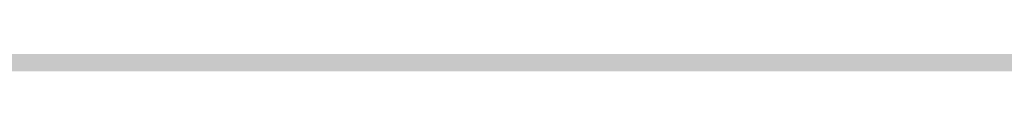
# Model space of a CAD drawing. Units: millimetres. Extents: x 0 to 2267, y 0 to 1823.
# Tile 72 of 256: x 1596.855 to 1600.369, y 1227.265 to 1227.284. Entities that reach past the tile are written whole.
import ezdxf

# ---------------------------------------------------------------- set-up
doc = ezdxf.new("R2010")
doc.units = ezdxf.units.MM
doc.header["$MEASUREMENT"] = 0
doc.layers.add('M-DIMS', color=2, linetype='Continuous', lineweight=25)
doc.layers.add('M-HATC', color=252, linetype='Continuous', lineweight=18)
doc.styles.get("Standard").update_dxf_attribs({"font": 'arial.ttf'})
doc.dimstyles.get("Standard").update_dxf_attribs({"dimtxt": 7, "dimasz": 4, "dimexe": 0.18, "dimexo": 0.0625, "dimgap": 0.09, "dimtad": 0, "dimdec": 0, "dimzin": 0, "dimdsep": 46, "dimtxsty": 'Standard', "dimcen": 0.09, "dimadec": 0, "dimazin": 0, "dimtfac": 1, "dimtdec": 0, "dimtofl": 0, "dimtmove": 0, "dimatfit": 3, "dimfxl": 1, "dimtolj": 1, "dimtzin": 0, "dimarcsym": 0})

# ---------------------------------------------------------------- blocks, each defined once
blk = doc.blocks.new('*D19')
at = {"layer": 'Defpoints', "color": 0, "transparency": 16777216}
for p in [(1605.3399, 1483.3044), (1445.5291, 1333.8851)]:
    blk.add_point(p, dxfattribs=at)
at = {"layer": 'M-DIMS', "color": 0, "lineweight": -2, "transparency": 16777216}
for p, q in [((1605.3399, 1483.2144), (1605.3399, 1483.3944)), ((1605.2499, 1483.3044), (1605.4299, 1483.3044)), ((1366.3244, 1259.8306), (1442.6072, 1331.1532))]:
    blk.add_line(p, q, dxfattribs=at)
at = {"layer": 'M-DIMS', "color": 0, "transparency": 16777216}
blk.add_solid([(1442.1519, 1331.6402), (1443.0625, 1330.6663), (1445.5291, 1333.8851)], dxfattribs=at)
at = {"layer": 'M-DIMS', "color": 0, "transparency": 16777216, "insert": (1349.6425, 1244.2335), "char_height": 7, "attachment_point": 5, "rotation": 43.0753}
blk.add_mtext('\\A1;2X R218.8', dxfattribs=at)

msp = doc.modelspace()

# ---------------------------------------------------------------- hatches: boundary and pattern name
at = {"layer": 'M-HATC'}
h = msp.add_hatch(color=256, dxfattribs=at)
h.dxf.hatch_style = 1
h.paths.add_polyline_path([(2055.771, 1603.062), (1381.0868, 1603.062), (1381.0868, 1598.062), (2055.771, 1598.062)])
h.paths.add_polyline_path([(2055.771, 1598.062), (1381.0868, 1598.062), (1381.0868, 1593.062), (2055.771, 1593.062)])
h.paths.add_polyline_path([(2051.3074, 1536.7609), (1385.5504, 1536.7609), (1385.5504, 1526.7609), (1387.5504, 1526.7609), (1388.5366, 1525.0528), (1385.3319, 1521.2335), (1385.3319, 1521.2226), (2050.2542, 1522.7491), (2048.3212, 1525.0528), (2049.3074, 1526.7609), (2051.3074, 1526.7609)])
edge = h.paths.add_edge_path()
edge.add_arc((1847.5345, 1379.1492), 135, 222.603061, 222.890851, ccw=False)
edge.add_line((1748.1663, 1287.7656), (1683.0921, 1287.7656))
edge.add_arc((1583.7239, 1379.1492), 135, 317.109149, 317.396939, ccw=False)
edge.add_arc((1678.9686, 1290.6707), 5, 222.8909, 317.1091, ccw=False)
edge.add_arc((1774.2133, 1379.1492), 135, 222.603061, 222.890851, ccw=False)
edge.add_line((1674.8451, 1287.7656), (1609.7709, 1287.7656))
edge.add_arc((1510.4027, 1379.1492), 135, 317.109149, 317.396939, ccw=False)
edge.add_arc((1605.6474, 1290.6707), 5, 222.8909, 317.1091, ccw=False)
edge.add_arc((1700.8921, 1379.1492), 135, 222.603061, 222.890851, ccw=False)
edge.add_line((1601.5239, 1287.7656), (1536.4497, 1287.7656))
edge.add_arc((1437.0815, 1379.1492), 135, 317.109149, 317.396939, ccw=False)
edge.add_arc((1532.3262, 1290.6707), 5, 222.8909, 317.1091, ccw=False)
edge.add_arc((1627.5709, 1379.1492), 135, 222.603061, 222.890851, ccw=False)
edge.add_line((1528.2027, 1287.7656), (1505.9289, 1287.7656))
edge.add_spline(control_points=[(1505.9289, 1287.7656), (1504.2622, 1287.7656), (1504.2622, 1282.7656), (1505.9289, 1282.7656)], knot_values=[0, 0, 0, 0, 5, 5, 5, 5], degree=3, periodic=0)
edge.add_line((1505.9289, 1282.7656), (1930.9289, 1282.7656))
edge.add_spline(control_points=[(1930.9289, 1282.7656), (1932.5956, 1282.7656), (1932.5956, 1287.7656), (1930.9289, 1287.7656)], knot_values=[0, 0, 0, 0, 5, 5, 5, 5], degree=3, periodic=0)
edge.add_line((1930.9289, 1287.7656), (1903.0557, 1287.7656))
edge.add_arc((1803.6875, 1379.1492), 135, 317.109149, 317.396939, ccw=False)
edge.add_arc((1898.9322, 1290.6707), 5, 222.8909, 317.1091, ccw=False)
edge.add_arc((1994.1769, 1379.1492), 135, 222.603061, 222.890851, ccw=False)
edge.add_line((1894.8087, 1287.7656), (1829.7345, 1287.7656))
edge.add_arc((1730.3663, 1379.1492), 135, 317.109149, 317.396939, ccw=False)
edge.add_arc((1825.611, 1290.6707), 5, 222.8909, 317.1091, ccw=False)
edge.add_arc((1920.8557, 1379.1492), 135, 222.603061, 222.890851, ccw=False)
edge.add_line((1821.4875, 1287.7656), (1756.4133, 1287.7656))
edge.add_arc((1657.0451, 1379.1492), 135, 317.109149, 317.396939, ccw=False)
edge.add_arc((1752.2898, 1290.6707), 5, 222.8909, 317.1091, ccw=False)
edge = h.paths.add_edge_path()
edge.add_spline(control_points=[(1843.4289, 1227.2475), (1845.0956, 1227.2475), (1845.0956, 1232.2475), (1843.4289, 1232.2475)], knot_values=[0, 0, 0, 0, 5, 5, 5, 5], degree=3, periodic=0)
edge.add_line((1843.4289, 1232.2475), (1593.4289, 1232.2475))
edge.add_spline(control_points=[(1593.4289, 1232.2475), (1591.7622, 1232.2475), (1591.7622, 1227.2475), (1593.4289, 1227.2475)], knot_values=[0, 0, 0, 0, 5, 5, 5, 5], degree=3, periodic=0)
edge.add_line((1593.4289, 1227.2475), (1843.4289, 1227.2475))
h.paths.add_polyline_path([(1905.9289, 1127.4171), (1530.9289, 1127.4171, 0.414214), (1520.9289, 1117.4171), (1530.9289, 1117.4171), (1915.9289, 1117.4171, 0.414214)])
edge = h.paths.add_edge_path()
edge.add_arc((1397.0858, 1498.4078), 12.7299, 90.78215, 190.87871, ccw=False)
edge.add_line((1396.912, 1511.1365), (1428.0097, 1511.3488))
edge.add_line((1428.0097, 1511.3488), (1433.0097, 1511.3488))
edge.add_line((1433.0097, 1511.3488), (1434.439, 1511.3488))
edge.add_arc((1419.474, 1498.0804), 20, 41.561, 74.08211)
edge.add_line((1424.9592, 1517.3135), (1399.9351, 1517.2561))
edge.add_spline(control_points=[(1399.9307, 1517.2561), (1399.884, 1517.2131), (1399.8328, 1517.1689), (1399.7774, 1517.1236)], knot_values=[11.567499, 11.567499, 11.567499, 11.567499, 11.814249, 11.814249, 11.814249, 11.814249], degree=3, periodic=0)
edge.add_spline(control_points=[(1399.6328, 1517.0099), (1399.5831, 1516.9721), (1399.5307, 1516.9338), (1399.4759, 1516.8947)], knot_values=[11.167718, 11.167718, 11.167718, 11.167718, 11.365188, 11.365188, 11.365188, 11.365188], degree=3, periodic=0)
edge.add_spline(control_points=[(1399.3398, 1516.8001), (1399.1514, 1516.6719), (1398.9384, 1516.5377), (1398.704, 1516.3994)], knot_values=[10.376405, 10.376405, 10.376405, 10.376405, 11.00994, 11.00994, 11.00994, 11.00994], degree=3, periodic=0)
edge.add_spline(control_points=[(1398.6572, 1516.3719), (1398.5789, 1516.326), (1398.4983, 1516.2797), (1398.4155, 1516.2331)], knot_values=[10.125175, 10.125175, 10.125175, 10.125175, 10.334406, 10.334406, 10.334406, 10.334406], degree=3, periodic=0)
edge.add_spline(control_points=[(1398.2642, 1516.1487), (1398.196, 1516.1111), (1398.1263, 1516.0732), (1398.0555, 1516.0351)], knot_values=[9.832246, 9.832246, 9.832246, 9.832246, 9.999658, 9.999658, 9.999658, 9.999658], degree=3, periodic=0)
edge.add_spline(control_points=[(1397.9987, 1516.0048), (1397.7312, 1515.8621), (1397.446, 1515.7171), (1397.1466, 1515.5714)], knot_values=[9.161808, 9.161808, 9.161808, 9.161808, 9.787769, 9.787769, 9.787769, 9.787769], degree=3, periodic=0)
edge.add_spline(control_points=[(1397.1466, 1515.5714), (1396.8418, 1515.423), (1396.5222, 1515.274), (1396.1914, 1515.1262)], knot_values=[8.524455, 8.524455, 8.524455, 8.524455, 9.161808, 9.161808, 9.161808, 9.161808], degree=3, periodic=0)
edge.add_spline(control_points=[(1396.0777, 1515.0756), (1395.9854, 1515.0348), (1395.8922, 1514.994), (1395.7983, 1514.9534)], knot_values=[8.275193, 8.275193, 8.275193, 8.275193, 8.451726, 8.451726, 8.451726, 8.451726], degree=3, periodic=0)
edge.add_spline(control_points=[(1395.6018, 1514.8691), (1395.4997, 1514.8257), (1395.3968, 1514.7824), (1395.2932, 1514.7394)], knot_values=[7.962917, 7.962917, 7.962917, 7.962917, 8.152764, 8.152764, 8.152764, 8.152764], degree=3, periodic=0)
edge.add_spline(control_points=[(1395.2116, 1514.7057), (1394.8278, 1514.5475), (1394.4345, 1514.3929), (1394.0364, 1514.2442)], knot_values=[7.21254, 7.21254, 7.21254, 7.21254, 7.913148, 7.913148, 7.913148, 7.913148], degree=3, periodic=0)
edge.add_spline(control_points=[(1394.0364, 1514.2442), (1393.7076, 1514.1214), (1393.3754, 1514.0027), (1393.0427, 1513.8895)], knot_values=[6.633733, 6.633733, 6.633733, 6.633733, 7.21254, 7.21254, 7.21254, 7.21254], degree=3, periodic=0)
edge.add_spline(control_points=[(1392.8214, 1513.815), (1392.7198, 1513.7812), (1392.6181, 1513.7479), (1392.5166, 1513.7152)], knot_values=[6.328796, 6.328796, 6.328796, 6.328796, 6.505493, 6.505493, 6.505493, 6.505493], degree=3, periodic=0)
edge.add_spline(control_points=[(1392.5166, 1513.7152), (1392.3187, 1513.6515), (1392.1212, 1513.59), (1391.9244, 1513.531)], knot_values=[5.984605, 5.984605, 5.984605, 5.984605, 6.328796, 6.328796, 6.328796, 6.328796], degree=3, periodic=0)
edge.add_spline(control_points=[(1391.7915, 1513.4915), (1391.3122, 1513.3501), (1390.8384, 1513.2239), (1390.3784, 1513.1171)], knot_values=[5.066697, 5.066697, 5.066697, 5.066697, 5.907055, 5.907055, 5.907055, 5.907055], degree=3, periodic=0)
edge.add_spline(control_points=[(1390.3784, 1513.1171), (1390.1797, 1513.071), (1389.9836, 1513.0284), (1389.7907, 1512.9899)], knot_values=[4.70367, 4.70367, 4.70367, 4.70367, 5.066695, 5.066695, 5.066695, 5.066695], degree=3, periodic=0)
edge.add_spline(control_points=[(1389.422, 1512.9204), (1389.2459, 1512.8892), (1389.0729, 1512.8617), (1388.9036, 1512.8381)], knot_values=[4.130571, 4.130571, 4.130571, 4.130571, 4.469816, 4.469816, 4.469816, 4.469816], degree=3, periodic=0)
edge.add_spline(control_points=[(1388.9036, 1512.8381), (1388.591, 1512.7946), (1388.2911, 1512.7644), (1388.0071, 1512.7494)], knot_values=[3.504031, 3.504031, 3.504031, 3.504031, 4.130571, 4.130571, 4.130571, 4.130571], degree=3, periodic=0)
edge.add_spline(control_points=[(1387.9356, 1512.7459), (1387.8538, 1512.7423), (1387.7733, 1512.74), (1387.6944, 1512.739)], knot_values=[3.268866, 3.268866, 3.268866, 3.268866, 3.451164, 3.451164, 3.451164, 3.451164], degree=3, periodic=0)
edge.add_spline(control_points=[(1387.3351, 1512.7443), (1387.2076, 1512.7499), (1387.0847, 1512.7597), (1386.967, 1512.7739)], knot_values=[2.670686, 2.670686, 2.670686, 2.670686, 2.984, 2.984, 2.984, 2.984], degree=3, periodic=0)
edge.add_spline(control_points=[(1386.8327, 1512.7922), (1386.8209, 1512.7941), (1386.8092, 1512.7959), (1386.7975, 1512.7979)], knot_values=[2.516981, 2.516981, 2.516981, 2.516981, 2.549528, 2.549528, 2.549528, 2.549528], degree=3, periodic=0)
edge.add_spline(control_points=[(1386.4526, 1512.8735), (1386.4257, 1512.881), (1386.3993, 1512.889), (1386.3733, 1512.8972)], knot_values=[2.095869, 2.095869, 2.095869, 2.095869, 2.17941, 2.17941, 2.17941, 2.17941], degree=3, periodic=0)
edge.add_spline(control_points=[(1386.0691, 1513.0189), (1386.0634, 1513.0217), (1386.0577, 1513.0246), (1386.052, 1513.0275)], knot_values=[1.72453, 1.72453, 1.72453, 1.72453, 1.745933, 1.745933, 1.745933, 1.745933], degree=3, periodic=0)
edge.add_arc((1399.474, 1498.0804), 20, 131.82432, 180)
edge.add_arc((1630.3336, 1505.5484), 250.9708, 181.705176, 236.427975)
edge.add_arc((1605.3399, 1483.3044), 218.7822, 238.660829, 243.34961)
edge.add_arc((1647.0911, 1510.3592), 262.8986, 183.129836, 237.853442, ccw=False)
h.paths.add_polyline_path([(1406.5369, 1391.9644, 0.149382), (1491.5506, 1296.4418, -0.129517)], flags=17)
edge = h.paths.add_edge_path()
edge.add_arc((2037.3838, 1498.0804), 20, 0, 48.26587)
edge.add_spline(control_points=[(2050.6973, 1513.0052), (2050.6512, 1512.9847), (2050.6034, 1512.9655), (2050.5539, 1512.9477)], knot_values=[1.835652, 1.835652, 1.835652, 1.835652, 2.000781, 2.000781, 2.000781, 2.000781], degree=3, periodic=0)
edge.add_spline(control_points=[(2050.4616, 1512.9166), (2050.479, 1512.9221), (2050.4963, 1512.9277), (2050.5133, 1512.9335)], knot_values=[2.045477, 2.045477, 2.045477, 2.045477, 2.101389, 2.101389, 2.101389, 2.101389], degree=3, periodic=0)
edge.add_spline(control_points=[(2050.129, 1512.8342), (2050.1984, 1512.8473), (2050.2657, 1512.8623), (2050.3308, 1512.8792)], knot_values=[2.237629, 2.237629, 2.237629, 2.237629, 2.435841, 2.435841, 2.435841, 2.435841], degree=3, periodic=0)
edge.add_spline(control_points=[(2050.0946, 1512.8278), (2050.1061, 1512.8299), (2050.1176, 1512.832), (2050.129, 1512.8342)], knot_values=[2.435841, 2.435841, 2.435841, 2.435841, 2.468321, 2.468321, 2.468321, 2.468321], degree=3, periodic=0)
edge.add_spline(control_points=[(2049.7843, 1512.7851), (2049.8552, 1512.7922), (2049.9243, 1512.8008), (2049.9917, 1512.8109)], knot_values=[2.563852, 2.563852, 2.563852, 2.563852, 2.748541, 2.748541, 2.748541, 2.748541], degree=3, periodic=0)
edge.add_spline(control_points=[(2049.4052, 1512.7617), (2049.5364, 1512.7653), (2049.6629, 1512.773), (2049.7843, 1512.7851)], knot_values=[2.748541, 2.748541, 2.748541, 2.748541, 3.064882, 3.064882, 3.064882, 3.064882], degree=3, periodic=0)
edge.add_spline(control_points=[(2049.1698, 1512.7597), (2049.2336, 1512.7591), (2049.2965, 1512.7594), (2049.3584, 1512.7606)], knot_values=[3.102309, 3.102309, 3.102309, 3.102309, 3.2503, 3.2503, 3.2503, 3.2503], degree=3, periodic=0)
edge.add_spline(control_points=[(2048.8573, 1512.7691), (2048.9638, 1512.7638), (2049.068, 1512.7606), (2049.1698, 1512.7597)], knot_values=[3.2503, 3.2503, 3.2503, 3.2503, 3.486069, 3.486069, 3.486069, 3.486069], degree=3, periodic=0)
edge.add_spline(control_points=[(2048.6924, 1512.7789), (2048.3729, 1512.8009), (2048.0345, 1512.8411), (2047.6817, 1512.897)], knot_values=[3.606429, 3.606429, 3.606429, 3.606429, 4.2989, 4.2989, 4.2989, 4.2989], degree=3, periodic=0)
edge.add_spline(control_points=[(2047.6817, 1512.897), (2047.5458, 1512.9185), (2047.4077, 1512.9424), (2047.2678, 1512.9685)], knot_values=[4.2989, 4.2989, 4.2989, 4.2989, 4.565769, 4.565769, 4.565769, 4.565769], degree=3, periodic=0)
edge.add_spline(control_points=[(2047.2678, 1512.9685), (2047.1449, 1512.9914), (2047.0207, 1513.016), (2046.8951, 1513.0422)], knot_values=[4.565769, 4.565769, 4.565769, 4.565769, 4.799971, 4.799971, 4.799971, 4.799971], degree=3, periodic=0)
edge.add_spline(control_points=[(2046.8951, 1513.0422), (2046.5286, 1513.1188), (2046.1513, 1513.209), (2045.7676, 1513.3107)], knot_values=[4.799971, 4.799971, 4.799971, 4.799971, 5.483718, 5.483718, 5.483718, 5.483718], degree=3, periodic=0)
edge.add_spline(control_points=[(2045.7676, 1513.3107), (2045.3724, 1513.4154), (2044.9704, 1513.5322), (2044.5662, 1513.6588)], knot_values=[5.483718, 5.483718, 5.483718, 5.483718, 6.187866, 6.187866, 6.187866, 6.187866], degree=3, periodic=0)
edge.add_spline(control_points=[(2044.5662, 1513.6588), (2044.4149, 1513.7061), (2044.2633, 1513.7549), (2044.1116, 1513.8048)], knot_values=[6.187866, 6.187866, 6.187866, 6.187866, 6.451551, 6.451551, 6.451551, 6.451551], degree=3, periodic=0)
edge.add_spline(control_points=[(2044.1116, 1513.8048), (2043.9967, 1513.8427), (2043.8817, 1513.8813), (2043.7668, 1513.9205)], knot_values=[6.451551, 6.451551, 6.451551, 6.451551, 6.651434, 6.651434, 6.651434, 6.651434], degree=3, periodic=0)
edge.add_spline(control_points=[(2043.7668, 1513.9205), (2043.3716, 1514.0554), (2042.9774, 1514.1979), (2042.5886, 1514.3458)], knot_values=[6.651434, 6.651434, 6.651434, 6.651434, 7.338879, 7.338879, 7.338879, 7.338879], degree=3, periodic=0)
edge.add_spline(control_points=[(2042.5886, 1514.3458), (2042.1643, 1514.5071), (2041.7465, 1514.6749), (2041.3409, 1514.846)], knot_values=[7.338879, 7.338879, 7.338879, 7.338879, 8.089209, 8.089209, 8.089209, 8.089209], degree=3, periodic=0)
edge.add_spline(control_points=[(2041.3409, 1514.846), (2041.1028, 1514.9465), (2040.869, 1515.0481), (2040.6405, 1515.1502)], knot_values=[8.089209, 8.089209, 8.089209, 8.089209, 8.529587, 8.529587, 8.529587, 8.529587], degree=3, periodic=0)
edge.add_spline(control_points=[(2040.51, 1515.2089), (2040.0824, 1515.4022), (2039.6747, 1515.5971), (2039.295, 1515.7894)], knot_values=[8.613818, 8.613818, 8.613818, 8.613818, 9.44571, 9.44571, 9.44571, 9.44571], degree=3, periodic=0)
edge.add_spline(control_points=[(2039.295, 1515.7894), (2039.0618, 1515.9075), (2038.8391, 1516.0246), (2038.6288, 1516.1398)], knot_values=[9.44571, 9.44571, 9.44571, 9.44571, 9.956404, 9.956404, 9.956404, 9.956404], degree=3, periodic=0)
edge.add_spline(control_points=[(2038.6288, 1516.1398), (2038.5187, 1516.2001), (2038.4121, 1516.2598), (2038.309, 1516.3189)], knot_values=[9.956404, 9.956404, 9.956404, 9.956404, 10.223542, 10.223542, 10.223542, 10.223542], degree=3, periodic=0)
edge.add_spline(control_points=[(2038.309, 1516.3189), (2038.2138, 1516.3735), (2038.1216, 1516.4276), (2038.0328, 1516.481)], knot_values=[10.223542, 10.223542, 10.223542, 10.223542, 10.47051, 10.47051, 10.47051, 10.47051], degree=3, periodic=0)
edge.add_spline(control_points=[(2038.0328, 1516.481), (2037.7855, 1516.6296), (2037.5639, 1516.773), (2037.3722, 1516.909)], knot_values=[10.47051, 10.47051, 10.47051, 10.47051, 11.15767, 11.15767, 11.15767, 11.15767], degree=3, periodic=0)
edge.add_spline(control_points=[(2037.3722, 1516.909), (2037.2789, 1516.9752), (2037.1927, 1517.0396), (2037.1142, 1517.102)], knot_values=[11.15767, 11.15767, 11.15767, 11.15767, 11.49227, 11.49227, 11.49227, 11.49227], degree=3, periodic=0)
edge.add_spline(control_points=[(2036.8564, 1517.3259), (2036.9148, 1517.2692), (2036.9814, 1517.2103), (2037.0557, 1517.1492)], knot_values=[11.577341, 11.577341, 11.577341, 11.577341, 11.91035, 11.91035, 11.91035, 11.91035], degree=3, periodic=0)
edge.add_spline(control_points=[(2036.8074, 1517.3748), (2036.823, 1517.3587), (2036.8393, 1517.3424), (2036.8564, 1517.3259)], knot_values=[11.91035, 11.91035, 11.91035, 11.91035, 12.007402, 12.007402, 12.007402, 12.007402], degree=3, periodic=0)
edge.add_spline(control_points=[(2036.7017, 1517.494), (2036.7104, 1517.483), (2036.7196, 1517.4719), (2036.7291, 1517.4606)], knot_values=[12.184155, 12.184155, 12.184155, 12.184155, 12.255409, 12.255409, 12.255409, 12.255409], degree=3, periodic=0)
edge.add_spline(control_points=[(2036.6159, 1517.6205), (2036.62, 1517.613), (2036.6243, 1517.6055), (2036.6289, 1517.5979)], knot_values=[12.487913, 12.487913, 12.487913, 12.487913, 12.541035, 12.541035, 12.541035, 12.541035], degree=3, periodic=0)
edge.add_spline(control_points=[(2036.5635, 1517.786), (2036.5637, 1517.7794), (2036.5642, 1517.7726), (2036.565, 1517.7658)], knot_values=[12.911761, 12.911761, 12.911761, 12.911761, 12.968286, 12.968286, 12.968286, 12.968286], degree=3, periodic=0)
edge.add_spline(control_points=[(2036.6166, 1517.9304), (2036.6125, 1517.9259), (2036.6086, 1517.9212), (2036.6049, 1517.9165)], knot_values=[13.382527, 13.382527, 13.382527, 13.382527, 13.433791, 13.433791, 13.433791, 13.433791], degree=3, periodic=0)
edge.add_spline(control_points=[(2036.749, 1518.017), (2036.7361, 1518.0116), (2036.7239, 1518.006), (2036.7124, 1518.0002)], knot_values=[13.726299, 13.726299, 13.726299, 13.726299, 13.809928, 13.809928, 13.809928, 13.809928], degree=3, periodic=0)
edge.add_spline(control_points=[(2036.8604, 1518.0528), (2036.8386, 1518.0474), (2036.8181, 1518.0416), (2036.7988, 1518.0353)], knot_values=[13.910887, 13.910887, 13.910887, 13.910887, 14.02153, 14.02153, 14.02153, 14.02153], degree=3, periodic=0)
edge.add_line((2036.9639, 1518.0804), (2032.3838, 1518.0804))
edge.add_line((2032.3838, 1518.0804), (2027.3838, 1518.0804))
edge.add_line((2027.3838, 1518.0804), (2022.3838, 1518.0804))
edge.add_line((2022.3838, 1518.0804), (2017.3838, 1518.0804))
edge.add_arc((2017.3838, 1498.0804), 20, 90, 138.439)
edge.add_line((2002.4188, 1511.3488), (2003.8481, 1511.3488))
edge.add_line((2003.8481, 1511.3488), (2008.8481, 1511.3488))
edge.add_line((2008.8481, 1511.3488), (2039.772, 1511.1377))
edge.add_arc((2039.772, 1498.4078), 12.7299, -10.87871, 90, ccw=False)
edge.add_arc((1789.7668, 1510.3592), 262.8986, 302.146558, 356.870164, ccw=False)
edge.add_arc((1831.5179, 1483.3044), 218.7822, 296.65039, 301.339171)
edge.add_arc((1806.5242, 1505.5484), 250.9708, 303.572025, 358.294824)
h.paths.add_polyline_path([(2030.321, 1391.9644, -0.129517), (1945.3072, 1296.4418, 0.149382)], flags=17)
edge = h.paths.add_edge_path()
edge.add_spline(control_points=[(2037.2464, 1518.0821), (2037.2898, 1518.081), (2037.3355, 1518.0804), (2037.3838, 1518.0804)], knot_values=[0.000012, 0.000012, 0.000012, 0.000012, 0.144754, 0.144754, 0.144754, 0.144754], degree=3, periodic=0)
edge.add_line((2037.3357, 1518.0804), (2037.0096, 1518.0804))
edge.add_spline(control_points=[(2037.0096, 1518.0804), (2036.9822, 1518.0768), (2036.956, 1518.0727), (2036.9312, 1518.0681)], knot_values=[14.13465, 14.13465, 14.13465, 14.13465, 14.247197, 14.247197, 14.247197, 14.247197], degree=3, periodic=0)
edge.add_spline(control_points=[(2036.9312, 1518.0681), (2036.9276, 1518.0674), (2036.9241, 1518.0667), (2036.9205, 1518.0661)], knot_values=[14.118315, 14.118315, 14.118315, 14.118315, 14.13465, 14.13465, 14.13465, 14.13465], degree=3, periodic=0)
edge.add_spline(control_points=[(2036.9205, 1518.0661), (2036.9118, 1518.0644), (2036.9032, 1518.0626), (2036.8948, 1518.0608)], knot_values=[14.078086, 14.078086, 14.078086, 14.078086, 14.118315, 14.118315, 14.118315, 14.118315], degree=3, periodic=0)
edge.add_spline(control_points=[(2036.8948, 1518.0608), (2036.883, 1518.0583), (2036.8716, 1518.0556), (2036.8604, 1518.0528)], knot_values=[14.02153, 14.02153, 14.02153, 14.02153, 14.078086, 14.078086, 14.078086, 14.078086], degree=3, periodic=0)
edge.add_spline(control_points=[(2036.8604, 1518.0528), (2036.8386, 1518.0474), (2036.8181, 1518.0416), (2036.7988, 1518.0353)], knot_values=[13.910887, 13.910887, 13.910887, 13.910887, 14.02153, 14.02153, 14.02153, 14.02153], degree=3, periodic=0)
edge.add_spline(control_points=[(2036.7988, 1518.0353), (2036.7981, 1518.035), (2036.7974, 1518.0348), (2036.7967, 1518.0346)], knot_values=[13.906906, 13.906906, 13.906906, 13.906906, 13.910887, 13.910887, 13.910887, 13.910887], degree=3, periodic=0)
edge.add_spline(control_points=[(2036.7967, 1518.0346), (2036.7882, 1518.0318), (2036.7799, 1518.0289), (2036.7719, 1518.0259)], knot_values=[13.857826, 13.857826, 13.857826, 13.857826, 13.906906, 13.906906, 13.906906, 13.906906], degree=3, periodic=0)
edge.add_spline(control_points=[(2036.7719, 1518.0259), (2036.764, 1518.023), (2036.7564, 1518.02), (2036.749, 1518.017)], knot_values=[13.809928, 13.809928, 13.809928, 13.809928, 13.857826, 13.857826, 13.857826, 13.857826], degree=3, periodic=0)
edge.add_spline(control_points=[(2036.749, 1518.017), (2036.7361, 1518.0116), (2036.7239, 1518.006), (2036.7124, 1518.0002)], knot_values=[13.726299, 13.726299, 13.726299, 13.726299, 13.809928, 13.809928, 13.809928, 13.809928], degree=3, periodic=0)
edge.add_spline(control_points=[(2036.7124, 1518.0002), (2036.7121, 1518), (2036.7118, 1517.9999), (2036.7115, 1517.9997)], knot_values=[13.723993, 13.723993, 13.723993, 13.723993, 13.726299, 13.726299, 13.726299, 13.726299], degree=3, periodic=0)
edge.add_spline(control_points=[(2036.7115, 1517.9997), (2036.7063, 1517.9971), (2036.7013, 1517.9944), (2036.6965, 1517.9917)], knot_values=[13.686536, 13.686536, 13.686536, 13.686536, 13.723993, 13.723993, 13.723993, 13.723993], degree=3, periodic=0)
edge.add_spline(control_points=[(2036.6965, 1517.9917), (2036.6919, 1517.9891), (2036.6874, 1517.9865), (2036.6831, 1517.9839)], knot_values=[13.651251, 13.651251, 13.651251, 13.651251, 13.686536, 13.686536, 13.686536, 13.686536], degree=3, periodic=0)
edge.add_spline(control_points=[(2036.6831, 1517.9839), (2036.6764, 1517.9798), (2036.67, 1517.9757), (2036.6639, 1517.9714)], knot_values=[13.596804, 13.596804, 13.596804, 13.596804, 13.651251, 13.651251, 13.651251, 13.651251], degree=3, periodic=0)
edge.add_spline(control_points=[(2036.6639, 1517.9714), (2036.6636, 1517.9712), (2036.6633, 1517.9709), (2036.6629, 1517.9707)], knot_values=[13.593956, 13.593956, 13.593956, 13.593956, 13.596804, 13.596804, 13.596804, 13.596804], degree=3, periodic=0)
edge.add_spline(control_points=[(2036.6629, 1517.9707), (2036.6603, 1517.9689), (2036.6577, 1517.967), (2036.6552, 1517.9651)], knot_values=[13.570322, 13.570322, 13.570322, 13.570322, 13.593956, 13.593956, 13.593956, 13.593956], degree=3, periodic=0)
edge.add_spline(control_points=[(2036.6552, 1517.9651), (2036.6525, 1517.9631), (2036.6499, 1517.9611), (2036.6474, 1517.9591)], knot_values=[13.545477, 13.545477, 13.545477, 13.545477, 13.570322, 13.570322, 13.570322, 13.570322], degree=3, periodic=0)
edge.add_spline(control_points=[(2036.6474, 1517.9591), (2036.6472, 1517.9589), (2036.6471, 1517.9588), (2036.6469, 1517.9587)], knot_values=[13.543931, 13.543931, 13.543931, 13.543931, 13.545477, 13.545477, 13.545477, 13.545477], degree=3, periodic=0)
edge.add_spline(control_points=[(2036.6469, 1517.9587), (2036.6412, 1517.9541), (2036.6358, 1517.9494), (2036.6307, 1517.9447)], knot_values=[13.488237, 13.488237, 13.488237, 13.488237, 13.543931, 13.543931, 13.543931, 13.543931], degree=3, periodic=0)
edge.add_spline(control_points=[(2036.6307, 1517.9447), (2036.6282, 1517.9423), (2036.6257, 1517.9399), (2036.6233, 1517.9374)], knot_values=[13.460307, 13.460307, 13.460307, 13.460307, 13.488237, 13.488237, 13.488237, 13.488237], degree=3, periodic=0)
edge.add_spline(control_points=[(2036.6233, 1517.9374), (2036.6215, 1517.9356), (2036.6198, 1517.9338), (2036.6181, 1517.932)], knot_values=[13.439712, 13.439712, 13.439712, 13.439712, 13.460307, 13.460307, 13.460307, 13.460307], degree=3, periodic=0)
edge.add_spline(control_points=[(2036.6181, 1517.932), (2036.6176, 1517.9315), (2036.6171, 1517.9309), (2036.6166, 1517.9304)], knot_values=[13.433791, 13.433791, 13.433791, 13.433791, 13.439712, 13.439712, 13.439712, 13.439712], degree=3, periodic=0)
edge.add_spline(control_points=[(2036.6166, 1517.9304), (2036.6125, 1517.9259), (2036.6086, 1517.9212), (2036.6049, 1517.9165)], knot_values=[13.382527, 13.382527, 13.382527, 13.382527, 13.433791, 13.433791, 13.433791, 13.433791], degree=3, periodic=0)
edge.add_spline(control_points=[(2036.6049, 1517.9165), (2036.6026, 1517.9135), (2036.6004, 1517.9104), (2036.5982, 1517.9074)], knot_values=[13.350017, 13.350017, 13.350017, 13.350017, 13.382527, 13.382527, 13.382527, 13.382527], degree=3, periodic=0)
edge.add_spline(control_points=[(2036.5982, 1517.9074), (2036.5972, 1517.9059), (2036.5962, 1517.9043), (2036.5952, 1517.9028)], knot_values=[13.333922, 13.333922, 13.333922, 13.333922, 13.350017, 13.350017, 13.350017, 13.350017], degree=3, periodic=0)
edge.add_spline(control_points=[(2036.5952, 1517.9028), (2036.5945, 1517.9018), (2036.5939, 1517.9009), (2036.5933, 1517.8999)], knot_values=[13.323828, 13.323828, 13.323828, 13.323828, 13.333922, 13.333922, 13.333922, 13.333922], degree=3, periodic=0)
edge.add_spline(control_points=[(2036.5933, 1517.8999), (2036.5905, 1517.8955), (2036.5879, 1517.8909), (2036.5855, 1517.8864)], knot_values=[13.277545, 13.277545, 13.277545, 13.277545, 13.323828, 13.323828, 13.323828, 13.323828], degree=3, periodic=0)
edge.add_spline(control_points=[(2036.5855, 1517.8864), (2036.5836, 1517.8827), (2036.5817, 1517.8789), (2036.5801, 1517.8751)], knot_values=[13.240119, 13.240119, 13.240119, 13.240119, 13.277545, 13.277545, 13.277545, 13.277545], degree=3, periodic=0)
edge.add_spline(control_points=[(2036.5801, 1517.8751), (2036.5795, 1517.8739), (2036.579, 1517.8727), (2036.5785, 1517.8715)], knot_values=[13.228211, 13.228211, 13.228211, 13.228211, 13.240119, 13.240119, 13.240119, 13.240119], degree=3, periodic=0)
edge.add_spline(control_points=[(2036.5785, 1517.8715), (2036.578, 1517.8702), (2036.5774, 1517.869), (2036.5769, 1517.8677)], knot_values=[13.215717, 13.215717, 13.215717, 13.215717, 13.228211, 13.228211, 13.228211, 13.228211], degree=3, periodic=0)
edge.add_spline(control_points=[(2036.5769, 1517.8677), (2036.5755, 1517.864), (2036.5741, 1517.8603), (2036.5729, 1517.8565)], knot_values=[13.179847, 13.179847, 13.179847, 13.179847, 13.215717, 13.215717, 13.215717, 13.215717], degree=3, periodic=0)
edge.add_spline(control_points=[(2036.5729, 1517.8565), (2036.5713, 1517.8515), (2036.5699, 1517.8464), (2036.5687, 1517.8413)], knot_values=[13.132017, 13.132017, 13.132017, 13.132017, 13.179847, 13.179847, 13.179847, 13.179847], degree=3, periodic=0)
edge.add_spline(control_points=[(2036.5687, 1517.8413), (2036.5684, 1517.8402), (2036.5682, 1517.8392), (2036.568, 1517.8382)], knot_values=[13.122482, 13.122482, 13.122482, 13.122482, 13.132017, 13.132017, 13.132017, 13.132017], degree=3, periodic=0)
edge.add_spline(control_points=[(2036.568, 1517.8382), (2036.5676, 1517.8363), (2036.5672, 1517.8345), (2036.5669, 1517.8327)], knot_values=[13.105592, 13.105592, 13.105592, 13.105592, 13.122482, 13.122482, 13.122482, 13.122482], degree=3, periodic=0)
edge.add_spline(control_points=[(2036.5669, 1517.8327), (2036.5662, 1517.8292), (2036.5657, 1517.8257), (2036.5652, 1517.8222)], knot_values=[13.074063, 13.074063, 13.074063, 13.074063, 13.105592, 13.105592, 13.105592, 13.105592], degree=3, periodic=0)
edge.add_spline(control_points=[(2036.5652, 1517.8222), (2036.5652, 1517.8222), (2036.5652, 1517.8222), (2036.5652, 1517.8222)], knot_values=[13.074043, 13.074043, 13.074043, 13.074043, 13.074063, 13.074063, 13.074063, 13.074063], degree=3, periodic=0)
edge.add_spline(control_points=[(2036.5652, 1517.8222), (2036.5644, 1517.8164), (2036.5639, 1517.8106), (2036.5636, 1517.8046)], knot_values=[13.021884, 13.021884, 13.021884, 13.021884, 13.074043, 13.074043, 13.074043, 13.074043], degree=3, periodic=0)
edge.add_spline(control_points=[(2036.5636, 1517.8046), (2036.5636, 1517.804), (2036.5636, 1517.8034), (2036.5635, 1517.8028)], knot_values=[13.01674, 13.01674, 13.01674, 13.01674, 13.021884, 13.021884, 13.021884, 13.021884], degree=3, periodic=0)
edge.add_spline(control_points=[(2036.5635, 1517.8028), (2036.5634, 1517.8005), (2036.5634, 1517.7982), (2036.5634, 1517.7958)], knot_values=[12.996438, 12.996438, 12.996438, 12.996438, 13.01674, 13.01674, 13.01674, 13.01674], degree=3, periodic=0)
edge.add_spline(control_points=[(2036.5634, 1517.7958), (2036.5633, 1517.7926), (2036.5634, 1517.7893), (2036.5635, 1517.786)], knot_values=[12.968286, 12.968286, 12.968286, 12.968286, 12.996438, 12.996438, 12.996438, 12.996438], degree=3, periodic=0)
edge.add_spline(control_points=[(2036.5635, 1517.786), (2036.5637, 1517.7794), (2036.5642, 1517.7726), (2036.565, 1517.7658)], knot_values=[12.911761, 12.911761, 12.911761, 12.911761, 12.968286, 12.968286, 12.968286, 12.968286], degree=3, periodic=0)
edge.add_spline(control_points=[(2036.565, 1517.7658), (2036.565, 1517.7657), (2036.565, 1517.7656), (2036.565, 1517.7656)], knot_values=[12.911017, 12.911017, 12.911017, 12.911017, 12.911761, 12.911761, 12.911761, 12.911761], degree=3, periodic=0)
edge.add_spline(control_points=[(2036.565, 1517.7656), (2036.5654, 1517.7625), (2036.5658, 1517.7593), (2036.5663, 1517.7562)], knot_values=[12.88528, 12.88528, 12.88528, 12.88528, 12.911017, 12.911017, 12.911017, 12.911017], degree=3, periodic=0)
edge.add_spline(control_points=[(2036.5663, 1517.7562), (2036.5667, 1517.7534), (2036.5672, 1517.7506), (2036.5677, 1517.7478)], knot_values=[12.862519, 12.862519, 12.862519, 12.862519, 12.88528, 12.88528, 12.88528, 12.88528], degree=3, periodic=0)
edge.add_spline(control_points=[(2036.5677, 1517.7478), (2036.5678, 1517.7474), (2036.5679, 1517.7469), (2036.568, 1517.7465)], knot_values=[12.858885, 12.858885, 12.858885, 12.858885, 12.862519, 12.862519, 12.862519, 12.862519], degree=3, periodic=0)
edge.add_spline(control_points=[(2036.568, 1517.7465), (2036.5692, 1517.7399), (2036.5707, 1517.7332), (2036.5724, 1517.7264)], knot_values=[12.8053, 12.8053, 12.8053, 12.8053, 12.858885, 12.858885, 12.858885, 12.858885], degree=3, periodic=0)
edge.add_spline(control_points=[(2036.5724, 1517.7264), (2036.5734, 1517.7226), (2036.5745, 1517.7187), (2036.5756, 1517.7149)], knot_values=[12.775176, 12.775176, 12.775176, 12.775176, 12.8053, 12.8053, 12.8053, 12.8053], degree=3, periodic=0)
edge.add_spline(control_points=[(2036.5756, 1517.7149), (2036.5763, 1517.7125), (2036.577, 1517.7102), (2036.5778, 1517.7078)], knot_values=[12.756759, 12.756759, 12.756759, 12.756759, 12.775176, 12.775176, 12.775176, 12.775176], degree=3, periodic=0)
edge.add_spline(control_points=[(2036.5778, 1517.7078), (2036.5781, 1517.7067), (2036.5784, 1517.7057), (2036.5787, 1517.7047)], knot_values=[12.748742, 12.748742, 12.748742, 12.748742, 12.756759, 12.756759, 12.756759, 12.756759], degree=3, periodic=0)
edge.add_spline(control_points=[(2036.5787, 1517.7047), (2036.5808, 1517.6983), (2036.5831, 1517.6919), (2036.5856, 1517.6854)], knot_values=[12.69959, 12.69959, 12.69959, 12.69959, 12.748742, 12.748742, 12.748742, 12.748742], degree=3, periodic=0)
edge.add_spline(control_points=[(2036.5856, 1517.6854), (2036.5876, 1517.68), (2036.5898, 1517.6746), (2036.5921, 1517.6692)], knot_values=[12.659038, 12.659038, 12.659038, 12.659038, 12.69959, 12.69959, 12.69959, 12.69959], degree=3, periodic=0)
edge.add_spline(control_points=[(2036.5921, 1517.6692), (2036.594, 1517.6648), (2036.5959, 1517.6605), (2036.5979, 1517.6561)], knot_values=[12.626806, 12.626806, 12.626806, 12.626806, 12.659038, 12.659038, 12.659038, 12.659038], degree=3, periodic=0)
edge.add_spline(control_points=[(2036.5979, 1517.6561), (2036.5984, 1517.6551), (2036.5989, 1517.6541), (2036.5993, 1517.6531)], knot_values=[12.619394, 12.619394, 12.619394, 12.619394, 12.626806, 12.626806, 12.626806, 12.626806], degree=3, periodic=0)
edge.add_spline(control_points=[(2036.5993, 1517.6531), (2036.6043, 1517.6424), (2036.6099, 1517.6315), (2036.6159, 1517.6205)], knot_values=[12.541039, 12.541039, 12.541039, 12.541039, 12.619394, 12.619394, 12.619394, 12.619394], degree=3, periodic=0)
edge.add_spline(control_points=[(2036.6159, 1517.6205), (2036.6159, 1517.6205), (2036.6159, 1517.6205), (2036.6159, 1517.6205)], knot_values=[12.541035, 12.541035, 12.541035, 12.541035, 12.541039, 12.541039, 12.541039, 12.541039], degree=3, periodic=0)
edge.add_spline(control_points=[(2036.6159, 1517.6205), (2036.62, 1517.613), (2036.6243, 1517.6055), (2036.6289, 1517.5979)], knot_values=[12.487913, 12.487913, 12.487913, 12.487913, 12.541035, 12.541035, 12.541035, 12.541035], degree=3, periodic=0)
edge.add_spline(control_points=[(2036.6289, 1517.5979), (2036.6326, 1517.5916), (2036.6365, 1517.5853), (2036.6406, 1517.5789)], knot_values=[12.443982, 12.443982, 12.443982, 12.443982, 12.487913, 12.487913, 12.487913, 12.487913], degree=3, periodic=0)
edge.add_spline(control_points=[(2036.6406, 1517.5789), (2036.6414, 1517.5776), (2036.6423, 1517.5763), (2036.6431, 1517.5749)], knot_values=[12.434996, 12.434996, 12.434996, 12.434996, 12.443982, 12.443982, 12.443982, 12.443982], degree=3, periodic=0)
edge.add_spline(control_points=[(2036.6431, 1517.5749), (2036.6531, 1517.5596), (2036.6639, 1517.5439), (2036.6756, 1517.528)], knot_values=[12.329647, 12.329647, 12.329647, 12.329647, 12.434996, 12.434996, 12.434996, 12.434996], degree=3, periodic=0)
edge.add_spline(control_points=[(2036.6756, 1517.528), (2036.6839, 1517.5168), (2036.6925, 1517.5055), (2036.7017, 1517.494)], knot_values=[12.255409, 12.255409, 12.255409, 12.255409, 12.329647, 12.329647, 12.329647, 12.329647], degree=3, periodic=0)
edge.add_spline(control_points=[(2036.7017, 1517.494), (2036.7104, 1517.483), (2036.7196, 1517.4719), (2036.7291, 1517.4606)], knot_values=[12.184155, 12.184155, 12.184155, 12.184155, 12.255409, 12.255409, 12.255409, 12.255409], degree=3, periodic=0)
edge.add_spline(control_points=[(2036.7291, 1517.4606), (2036.7436, 1517.4435), (2036.759, 1517.4262), (2036.7753, 1517.4085)], knot_values=[12.075961, 12.075961, 12.075961, 12.075961, 12.184155, 12.184155, 12.184155, 12.184155], degree=3, periodic=0)
edge.add_spline(control_points=[(2036.7753, 1517.4085), (2036.7763, 1517.4075), (2036.7773, 1517.4064), (2036.7783, 1517.4054)], knot_values=[12.069502, 12.069502, 12.069502, 12.069502, 12.075961, 12.075961, 12.075961, 12.075961], degree=3, periodic=0)
edge.add_spline(control_points=[(2036.7783, 1517.4054), (2036.7877, 1517.3953), (2036.7974, 1517.385), (2036.8074, 1517.3748)], knot_values=[12.007402, 12.007402, 12.007402, 12.007402, 12.069502, 12.069502, 12.069502, 12.069502], degree=3, periodic=0)
edge.add_spline(control_points=[(2036.8074, 1517.3748), (2036.823, 1517.3587), (2036.8393, 1517.3424), (2036.8564, 1517.3259)], knot_values=[11.91035, 11.91035, 11.91035, 11.91035, 12.007402, 12.007402, 12.007402, 12.007402], degree=3, periodic=0)
edge.add_spline(control_points=[(2036.8564, 1517.3259), (2036.9148, 1517.2692), (2036.9814, 1517.2103), (2037.0557, 1517.1492)], knot_values=[11.577341, 11.577341, 11.577341, 11.577341, 11.91035, 11.91035, 11.91035, 11.91035], degree=3, periodic=0)
edge.add_spline(control_points=[(2037.0557, 1517.1492), (2037.0747, 1517.1336), (2037.0942, 1517.1179), (2037.1142, 1517.102)], knot_values=[11.49227, 11.49227, 11.49227, 11.49227, 11.577341, 11.577341, 11.577341, 11.577341], degree=3, periodic=0)
edge.add_spline(control_points=[(2037.1142, 1517.102), (2037.1927, 1517.0396), (2037.2789, 1516.9752), (2037.3722, 1516.909)], knot_values=[11.15767, 11.15767, 11.15767, 11.15767, 11.49227, 11.49227, 11.49227, 11.49227], degree=3, periodic=0)
edge.add_spline(control_points=[(2037.3722, 1516.909), (2037.5639, 1516.773), (2037.7855, 1516.6296), (2038.0328, 1516.481)], knot_values=[10.47051, 10.47051, 10.47051, 10.47051, 11.15767, 11.15767, 11.15767, 11.15767], degree=3, periodic=0)
edge.add_spline(control_points=[(2038.0328, 1516.481), (2038.1216, 1516.4276), (2038.2138, 1516.3735), (2038.309, 1516.3189)], knot_values=[10.223542, 10.223542, 10.223542, 10.223542, 10.47051, 10.47051, 10.47051, 10.47051], degree=3, periodic=0)
edge.add_spline(control_points=[(2038.309, 1516.3189), (2038.4121, 1516.2598), (2038.5187, 1516.2001), (2038.6288, 1516.1398)], knot_values=[9.956404, 9.956404, 9.956404, 9.956404, 10.223542, 10.223542, 10.223542, 10.223542], degree=3, periodic=0)
edge.add_spline(control_points=[(2038.6288, 1516.1398), (2038.8391, 1516.0246), (2039.0618, 1515.9075), (2039.295, 1515.7894)], knot_values=[9.44571, 9.44571, 9.44571, 9.44571, 9.956404, 9.956404, 9.956404, 9.956404], degree=3, periodic=0)
edge.add_spline(control_points=[(2039.295, 1515.7894), (2039.6747, 1515.5971), (2040.0824, 1515.4022), (2040.51, 1515.2089)], knot_values=[8.613818, 8.613818, 8.613818, 8.613818, 9.44571, 9.44571, 9.44571, 9.44571], degree=3, periodic=0)
edge.add_spline(control_points=[(2040.51, 1515.2089), (2040.5533, 1515.1893), (2040.5968, 1515.1697), (2040.6405, 1515.1502)], knot_values=[8.529587, 8.529587, 8.529587, 8.529587, 8.613818, 8.613818, 8.613818, 8.613818], degree=3, periodic=0)
edge.add_spline(control_points=[(2040.6405, 1515.1502), (2040.869, 1515.0481), (2041.1028, 1514.9465), (2041.3409, 1514.846)], knot_values=[8.089209, 8.089209, 8.089209, 8.089209, 8.529587, 8.529587, 8.529587, 8.529587], degree=3, periodic=0)
edge.add_spline(control_points=[(2041.3409, 1514.846), (2041.7465, 1514.6749), (2042.1643, 1514.5071), (2042.5886, 1514.3458)], knot_values=[7.338879, 7.338879, 7.338879, 7.338879, 8.089209, 8.089209, 8.089209, 8.089209], degree=3, periodic=0)
edge.add_spline(control_points=[(2042.5886, 1514.3458), (2042.9774, 1514.1979), (2043.3716, 1514.0554), (2043.7668, 1513.9205)], knot_values=[6.651434, 6.651434, 6.651434, 6.651434, 7.338879, 7.338879, 7.338879, 7.338879], degree=3, periodic=0)
edge.add_spline(control_points=[(2043.7668, 1513.9205), (2043.8817, 1513.8813), (2043.9967, 1513.8427), (2044.1116, 1513.8048)], knot_values=[6.451551, 6.451551, 6.451551, 6.451551, 6.651434, 6.651434, 6.651434, 6.651434], degree=3, periodic=0)
edge.add_spline(control_points=[(2044.1116, 1513.8048), (2044.2633, 1513.7549), (2044.4149, 1513.7061), (2044.5662, 1513.6588)], knot_values=[6.187866, 6.187866, 6.187866, 6.187866, 6.451551, 6.451551, 6.451551, 6.451551], degree=3, periodic=0)
edge.add_spline(control_points=[(2044.5662, 1513.6588), (2044.9704, 1513.5322), (2045.3724, 1513.4154), (2045.7676, 1513.3107)], knot_values=[5.483718, 5.483718, 5.483718, 5.483718, 6.187866, 6.187866, 6.187866, 6.187866], degree=3, periodic=0)
edge.add_spline(control_points=[(2045.7676, 1513.3107), (2046.1513, 1513.209), (2046.5286, 1513.1188), (2046.8951, 1513.0422)], knot_values=[4.799971, 4.799971, 4.799971, 4.799971, 5.483718, 5.483718, 5.483718, 5.483718], degree=3, periodic=0)
edge.add_spline(control_points=[(2046.8951, 1513.0422), (2047.0207, 1513.016), (2047.1449, 1512.9914), (2047.2678, 1512.9685)], knot_values=[4.565769, 4.565769, 4.565769, 4.565769, 4.799971, 4.799971, 4.799971, 4.799971], degree=3, periodic=0)
edge.add_spline(control_points=[(2047.2678, 1512.9685), (2047.4077, 1512.9424), (2047.5458, 1512.9185), (2047.6817, 1512.897)], knot_values=[4.2989, 4.2989, 4.2989, 4.2989, 4.565769, 4.565769, 4.565769, 4.565769], degree=3, periodic=0)
edge.add_spline(control_points=[(2047.6817, 1512.897), (2048.0345, 1512.8411), (2048.3729, 1512.8009), (2048.6924, 1512.7789)], knot_values=[3.606429, 3.606429, 3.606429, 3.606429, 4.2989, 4.2989, 4.2989, 4.2989], degree=3, periodic=0)
edge.add_spline(control_points=[(2048.6924, 1512.7789), (2048.7479, 1512.7751), (2048.8029, 1512.7718), (2048.8573, 1512.7691)], knot_values=[3.486069, 3.486069, 3.486069, 3.486069, 3.606429, 3.606429, 3.606429, 3.606429], degree=3, periodic=0)
edge.add_spline(control_points=[(2048.8573, 1512.7691), (2048.9638, 1512.7638), (2049.068, 1512.7606), (2049.1698, 1512.7597)], knot_values=[3.2503, 3.2503, 3.2503, 3.2503, 3.486069, 3.486069, 3.486069, 3.486069], degree=3, periodic=0)
edge.add_spline(control_points=[(2049.1698, 1512.7597), (2049.2336, 1512.7591), (2049.2965, 1512.7594), (2049.3584, 1512.7606)], knot_values=[3.102309, 3.102309, 3.102309, 3.102309, 3.2503, 3.2503, 3.2503, 3.2503], degree=3, periodic=0)
edge.add_spline(control_points=[(2049.3584, 1512.7606), (2049.3741, 1512.7609), (2049.3897, 1512.7613), (2049.4052, 1512.7617)], knot_values=[3.064882, 3.064882, 3.064882, 3.064882, 3.102309, 3.102309, 3.102309, 3.102309], degree=3, periodic=0)
edge.add_spline(control_points=[(2049.4052, 1512.7617), (2049.5364, 1512.7653), (2049.6629, 1512.773), (2049.7843, 1512.7851)], knot_values=[2.748541, 2.748541, 2.748541, 2.748541, 3.064882, 3.064882, 3.064882, 3.064882], degree=3, periodic=0)
edge.add_spline(control_points=[(2049.7843, 1512.7851), (2049.8552, 1512.7922), (2049.9243, 1512.8008), (2049.9917, 1512.8109)], knot_values=[2.563852, 2.563852, 2.563852, 2.563852, 2.748541, 2.748541, 2.748541, 2.748541], degree=3, periodic=0)
edge.add_spline(control_points=[(2049.9917, 1512.8109), (2050.0265, 1512.8161), (2050.0608, 1512.8218), (2050.0946, 1512.8278)], knot_values=[2.468321, 2.468321, 2.468321, 2.468321, 2.563852, 2.563852, 2.563852, 2.563852], degree=3, periodic=0)
edge.add_spline(control_points=[(2050.0946, 1512.8278), (2050.1061, 1512.8299), (2050.1176, 1512.832), (2050.129, 1512.8342)], knot_values=[2.435841, 2.435841, 2.435841, 2.435841, 2.468321, 2.468321, 2.468321, 2.468321], degree=3, periodic=0)
edge.add_spline(control_points=[(2050.129, 1512.8342), (2050.1984, 1512.8473), (2050.2657, 1512.8623), (2050.3308, 1512.8792)], knot_values=[2.237629, 2.237629, 2.237629, 2.237629, 2.435841, 2.435841, 2.435841, 2.435841], degree=3, periodic=0)
edge.add_spline(control_points=[(2050.3308, 1512.8792), (2050.3754, 1512.8908), (2050.4191, 1512.9032), (2050.4616, 1512.9166)], knot_values=[2.101389, 2.101389, 2.101389, 2.101389, 2.237629, 2.237629, 2.237629, 2.237629], degree=3, periodic=0)
edge.add_spline(control_points=[(2050.4616, 1512.9166), (2050.479, 1512.9221), (2050.4963, 1512.9277), (2050.5133, 1512.9335)], knot_values=[2.045477, 2.045477, 2.045477, 2.045477, 2.101389, 2.101389, 2.101389, 2.101389], degree=3, periodic=0)
edge.add_spline(control_points=[(2050.5133, 1512.9335), (2050.527, 1512.9382), (2050.5405, 1512.9429), (2050.5539, 1512.9477)], knot_values=[2.000781, 2.000781, 2.000781, 2.000781, 2.045477, 2.045477, 2.045477, 2.045477], degree=3, periodic=0)
edge.add_spline(control_points=[(2050.5539, 1512.9477), (2050.6034, 1512.9655), (2050.6512, 1512.9847), (2050.6973, 1513.0052)], knot_values=[1.835652, 1.835652, 1.835652, 1.835652, 2.000781, 2.000781, 2.000781, 2.000781], degree=3, periodic=0)
edge.add_arc((2037.3838, 1498.0804), 20, 48.26587, 90.12993)
edge = h.paths.add_edge_path(flags=16)
edge.add_spline(control_points=[(1386.1389, 1512.9859), (1388.92, 1511.7395), (1398.0387, 1515.5187), (1399.9307, 1517.2561)], knot_values=[1.831046, 1.831046, 1.831046, 1.831046, 11.814249, 11.814249, 11.814249, 11.814249], degree=3, periodic=0)
edge.add_line((1399.9307, 1517.2561), (1393.7435, 1517.2419))
edge.add_arc((1399.474, 1498.0804), 20, 106.6501, 131.8173)

# ---------------------------------------------------------------- dimensions: what is measured, and where the dimension line sits
at = {"layer": 'M-DIMS'}
dim = msp.add_radius_dim(center=(1605.3399, 1483.3044), mpoint=(1445.5291, 1333.8851), text='2X <>', dimstyle='Standard', override={"dimdec": 1, "dimlfac": 1, "dimrnd": 0, "dimzin": 0, "dimdsep": 46, "dimlunit": 2}, dxfattribs=at)
dim.commit()
dim.dimension.update_dxf_attribs({"geometry": '*D19', "text_midpoint": (1349.6425, 1244.2335), "dimtype": 164})

doc.saveas('drawing.dxf')
